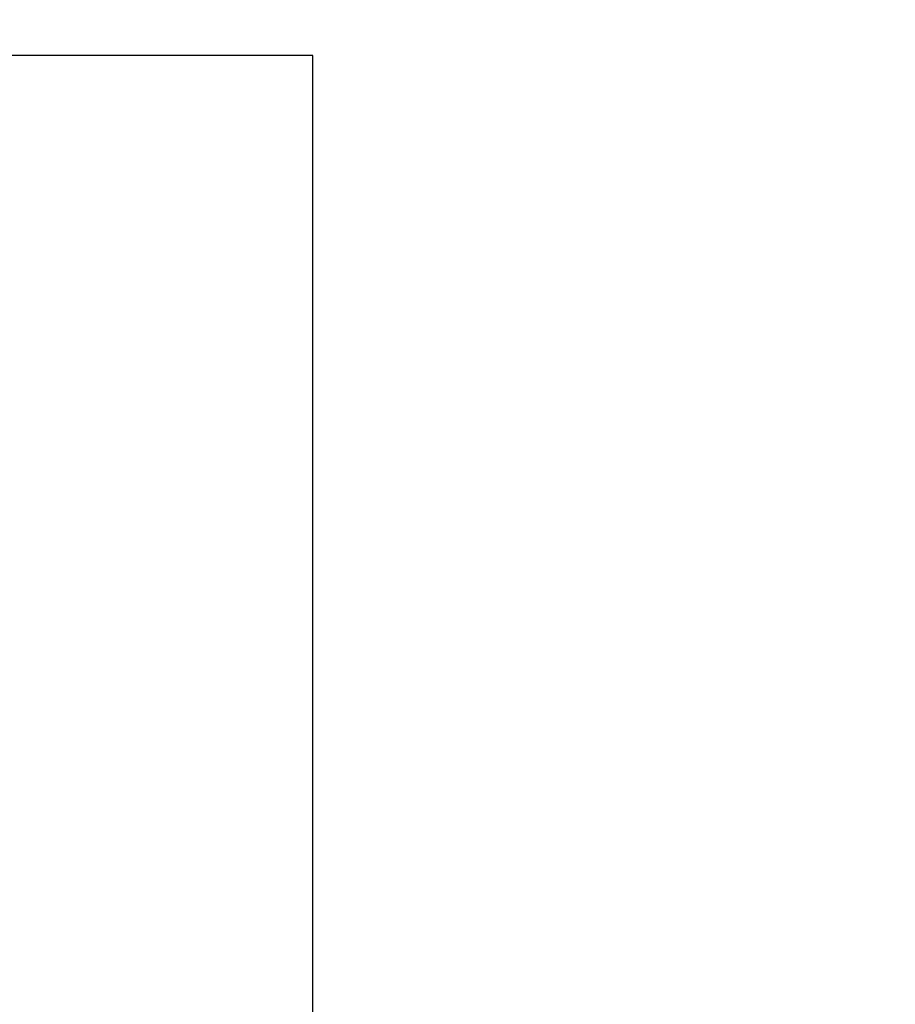
# Model space of a CAD drawing. Units: inches. Extents: x -1198 to -69, y -512 to 437.
# Tile 38 of 50: x -622.66 to -609.95, y 171.46 to 185.75. Entities that reach past the tile are written whole.
import ezdxf

# ---------------------------------------------------------------- set-up
doc = ezdxf.new("R2010")
doc.units = ezdxf.units.IN
doc.header["$MEASUREMENT"] = 0
doc.layers.add('A-ANNO-DIMS', color=2, linetype='Continuous', lineweight=18)
doc.layers.add('A-FLOR-CASE', color=7, linetype='Continuous', lineweight=25)
doc.styles.get("Standard").update_dxf_attribs({"font": 'arial.ttf'})
doc.dimstyles.get("Standard").update_dxf_attribs({"dimtxt": 6, "dimasz": 6, "dimexe": 0.18, "dimexo": 0.0625, "dimgap": 0.09, "dimtad": 0, "dimtih": 1, "dimtoh": 1, "dimdec": 0, "dimzin": 0, "dimdsep": 46, "dimlunit": 4, "dimtxsty": 'Standard', "dimblk": 'OBLIQUE', "dimcen": 0.09, "dimadec": 0, "dimazin": 0, "dimtfac": 1, "dimtdec": 0, "dimtofl": 0, "dimtmove": 0, "dimatfit": 3, "dimfxl": 1, "dimtolj": 1, "dimtzin": 0, "dimarcsym": 0})

# ---------------------------------------------------------------- blocks, each defined once
blk = doc.blocks.new('COUNTER-L')
at = {"ltscale": 10}
for p, q in [((49.349, 24), (0, 24)), ((49.349, 0), (49.349, 24))]:
    blk.add_line(p, q, dxfattribs=at)
blk = doc.blocks.new('_Oblique')
at = {"color": 0, "linetype": 'ByBlock', "lineweight": -2}
blk.add_line((-0.5, -0.5), (0.5, 0.5), dxfattribs=at)
blk = doc.blocks.new('*D56')
at = {"layer": 'A-ANNO-DIMS', "color": 0, "lineweight": -2, "ltscale": 10, "transparency": 16777216}
for p, q in [((-618.339, 257.228), (-603.822, 257.228)), ((-604.002, 257.228), (-604.002, 212.422)), ((-604.002, 161.228), (-604.002, 206.033)), ((-618.339, 161.228), (-603.822, 161.228))]:
    blk.add_line(p, q, dxfattribs=at)
at = {"layer": 'DEFPOINTS', "color": 0, "ltscale": 10, "transparency": 16777216}
for p in [(-618.402, 257.228), (-604.002, 257.228), (-618.402, 161.228)]:
    blk.add_point(p, dxfattribs=at)
at = {"layer": 'A-ANNO-DIMS', "color": 0, "lineweight": -2, "ltscale": 10, "transparency": 16777216, "xscale": 6, "yscale": 6, "zscale": 6}
for p, rotation in [((-604.002, 257.228), 90), ((-604.002, 161.228), 270)]:
    blk.add_blockref('_Oblique', p, dxfattribs=dict(at, rotation=rotation))
at = {"layer": 'A-ANNO-DIMS', "color": 0, "ltscale": 10, "transparency": 16777216, "insert": (-604.002, 209.228), "char_height": 6, "attachment_point": 5}
blk.add_mtext('\\A1;COUNTER 96 TYP.', dxfattribs=at)

msp = doc.modelspace()

# ---------------------------------------------------------------- block references
at = {"layer": 'A-FLOR-CASE'}
msp.add_blockref('COUNTER-L', (-667.751, 161.228), dxfattribs=at)

# ---------------------------------------------------------------- dimensions: what is measured, and where the dimension line sits
at = {"layer": 'A-ANNO-DIMS', "ltscale": 10}
dim = msp.add_linear_dim(base=(-604.0019, 257.2277), p1=(-618.4019, 161.2277), p2=(-618.4019, 257.2277), angle=90, text='COUNTER <> TYP.', dimstyle='Standard', override={"dimdec": 0, "dimlfac": 1, "dimrnd": 0, "dimzin": 0, "dimdsep": 46, "dimlunit": 2}, dxfattribs=at)
dim.commit()
dim.dimension.update_dxf_attribs({"geometry": '*D56', "text_midpoint": (-604.0019, 209.2277)})

doc.saveas('drawing.dxf')
